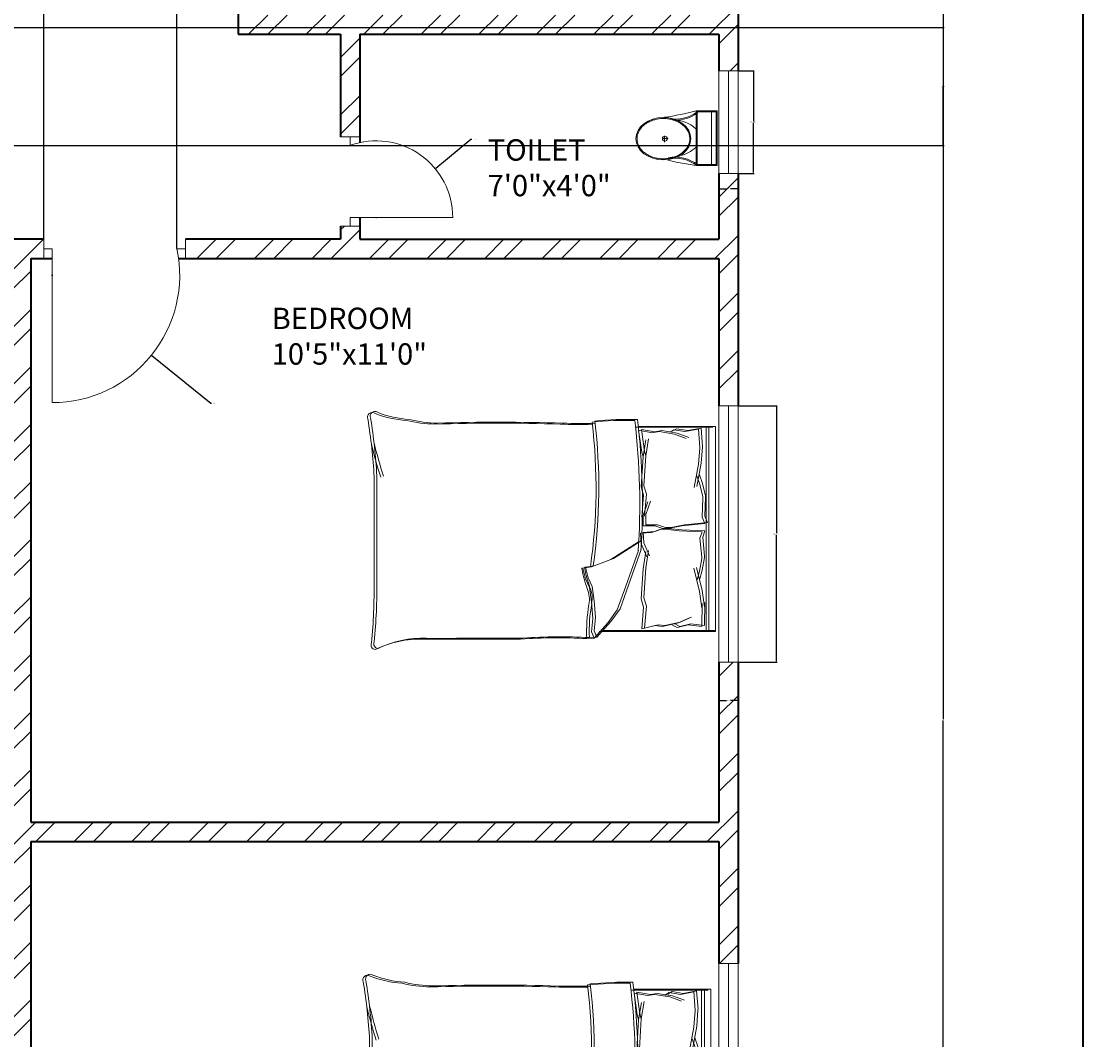
# Model space of a CAD drawing. Units: inches. Extents: x 2008 to 2657, y 1077 to 2165.
# Tile 14 of 16: x 2409 to 2657, y 1567 to 1805. Entities that reach past the tile are written whole.
import ezdxf

# ---------------------------------------------------------------- set-up
doc = ezdxf.new("R2010")
doc.units = ezdxf.units.IN
for name, color, linetype, lineweight in [('A-ANNO-DIMS', 2, 'Continuous', 18), ('A-ANNO-TTLB', 7, 'Continuous', 35), ('A-AREA-IDEN', 4, 'Continuous', 18), ('A-DOOR', 11, 'Continuous', 18), ('A-FLOR-FIXT', 8, 'Continuous', 18), ('A-FURN', 8, 'Continuous', 13), ('A-GLAZ', 191, 'Continuous', 18), ('A-WALL', 7, 'Continuous', 35)]:
    doc.layers.add(name, color=color, linetype=linetype, lineweight=lineweight)
doc.layers.add('A-WALL-PATT', color=30, linetype='Continuous', lineweight=13, true_color=0xf8991e)
doc.styles.get("Standard").update_dxf_attribs({"font": 'arial.ttf'})
doc.dimstyles.get("Standard").update_dxf_attribs({"dimtxt": 0.18, "dimasz": 0.18, "dimexe": 0.18, "dimexo": 0.0625, "dimgap": 0.09, "dimtad": 0, "dimtih": 1, "dimtoh": 1, "dimdec": 4, "dimzin": 0, "dimdsep": 46, "dimtxsty": 'Standard', "dimcen": 0.09, "dimadec": 0, "dimazin": 0, "dimtfac": 1, "dimtdec": 4, "dimtofl": 0, "dimtmove": 0, "dimatfit": 3, "dimfxl": 1, "dimtolj": 1, "dimtzin": 0, "dimarcsym": 0})

# ---------------------------------------------------------------- blocks, each defined once
blk = doc.blocks.new('A$C31115884')
for p, q in [((258, 466), (258, 523)), ((283, 498), (223, 498)), ((0, 200), (0, 0)), ((520, 200), (0, 200)), ((10, 190), (10, 10)), ((510, 190), (10, 190)), ((510, 10), (510, 190)), ((520, 0), (520, 200)), ((510, 54), (0, 54)), ((10, 10), (510, 10)), ((0, 0), (520, 0))]:
    blk.add_line(p, q)
blk.add_circle((256, 496), 23.6)
for centre, radius, start, end in [((2778, -205), 2807, 165.4549, 171.7133), ((-295, 403), 365, 324.2091, 9.3499), ((-295, 403), 375, 324.2091, 9.3499), ((139, 406), 293, 315.8436, 2.6563), ((806, 403), 375, 179.2036, 215.7909), ((806, 403), 365, 170.6501, 215.7909), ((3237, 905), 2807, 188.2867, 194.5451), ((384, 406), 293, 190.2774, 224.1564)]:
    blk.add_arc(centre, radius, start, end)
blk.add_ellipse((256, 510), major_axis=(0, -261), ratio=0.772727)
blk.add_open_spline([(256, 259), (263, 259), (270, 260), (288, 262), (299, 265), (320, 273), (330, 278), (350, 291), (360, 299), (378, 316), (386, 326), (402, 347), (409, 358), (421, 383), (427, 395), (436, 422), (440, 436), (445, 465), (447, 480), (448, 509), (448, 524), (445, 553), (443, 568), (436, 596), (432, 610), (422, 636), (416, 649), (402, 672), (395, 683), (379, 703), (370, 712), (351, 728), (341, 735), (321, 746), (310, 751), (289, 757), (278, 759), (256, 761), (245, 761), (223, 757), (212, 754), (191, 746), (181, 741), (161, 728), (151, 720), (133, 703), (125, 693), (110, 672), (103, 660), (90, 636), (85, 623), (76, 596), (72, 582), (67, 553), (66, 538), (64, 509), (65, 494), (68, 465), (70, 450), (77, 422), (81, 408), (91, 382), (97, 370), (111, 346), (118, 335), (135, 316), (144, 307), (162, 291), (172, 284), (193, 273), (203, 269), (225, 262), (236, 260), (250, 259), (253, 259), (256, 259)], degree=3, knots=[0, 0, 0, 0, 0.110105, 0.110105, 0.285049, 0.285049, 0.459994, 0.459994, 0.634938, 0.634938, 0.809882, 0.809882, 0.984827, 0.984827, 1.159771, 1.159771, 1.334715, 1.334715, 1.50966, 1.50966, 1.684604, 1.684604, 1.859549, 1.859549, 2.034493, 2.034493, 2.209437, 2.209437, 2.384382, 2.384382, 2.559326, 2.559326, 2.73427, 2.73427, 2.909215, 2.909215, 3.084159, 3.084159, 3.259103, 3.259103, 3.434048, 3.434048, 3.608992, 3.608992, 3.783936, 3.783936, 3.958881, 3.958881, 4.133825, 4.133825, 4.30877, 4.30877, 4.483714, 4.483714, 4.658658, 4.658658, 4.833603, 4.833603, 5.008547, 5.008547, 5.183491, 5.183491, 5.358436, 5.358436, 5.53338, 5.53338, 5.708324, 5.708324, 5.883269, 5.883269, 6.058213, 6.058213, 6.233158, 6.233158, 6.283185, 6.283185, 6.283185, 6.283185])
blk = doc.blocks.new('BED-DOUBLE')
for p, q in [((27.75, 52.87), (24.5, 49.16)), ((27.75, 52.87), (24.5, 49.16)), ((28.39, 53.1), (25.14, 49.39)), ((28.39, 53.1), (25.14, 49.39)), ((29.49, 52.95), (27.75, 52.87, 3.87)), ((29.49, 52.95), (27.75, 52.87, 3.87)), ((28.37, 51.33), (27.75, 52.87)), ((28.37, 51.33), (27.75, 52.87)), ((30.13, 53.18), (28.39, 53.1, 3.87)), ((30.13, 53.18), (28.39, 53.1, 3.87)), ((29, 51.56), (28.39, 53.1)), ((29, 51.56), (28.39, 53.1)), ((0, 51.49), (0.64, 51.49)), ((0, 3.48), (0, 51.49)), ((0, 51.27), (26.61, 51.27)), ((0, 51.27), (26.61, 51.27)), ((0.64, 51.49), (27.25, 51.49)), ((0.64, 51.49), (27.25, 51.49)), ((1.53, 3.48), (1.53, 51.27)), ((1.53, 3.48), (1.53, 51.27)), ((2.17, 3.7), (2.17, 51.49)), ((2.17, 3.7), (2.17, 51.49)), ((2.56, 50.11), (2.46, 44.71)), ((2.56, 50.11), (2.46, 44.71)), ((2.56, 50.11), (5.77, 49.73)), ((2.56, 50.11), (5.77, 49.73)), ((3.2, 50.34), (3.1, 44.94)), ((3.2, 50.34), (3.1, 44.94)), ((3.2, 50.34), (6.41, 49.96)), ((3.2, 50.34), (6.41, 49.96)), ((5.77, 49.73), (8.34, 50.33)), ((5.77, 49.73), (8.34, 50.33)), ((6.41, 49.96), (8.98, 50.56)), ((6.41, 49.96), (8.98, 50.56)), ((11.83, 50.11), (8.26, 49.31)), ((11.83, 50.11), (8.26, 49.31)), ((8.34, 50.33), (9.38, 49.82)), ((8.34, 50.33), (9.38, 49.81)), ((12.47, 50.34), (8.9, 49.54)), ((12.47, 50.34), (8.9, 49.54)), ((8.98, 50.56), (10.02, 50.04)), ((8.98, 50.56), (10.02, 50.04)), ((13.43, 49.92), (11.83, 50.11)), ((13.43, 49.92), (11.83, 50.11)), ((14.07, 50.15), (12.47, 50.34)), ((14.07, 50.15), (12.47, 50.34)), ((16.57, 50.7), (13.43, 49.92)), ((16.57, 50.7), (13.43, 49.92)), ((17.21, 50.93), (14.07, 50.15)), ((17.21, 50.93), (14.07, 50.15)), ((16.17, 45.57), (16.57, 50.7)), ((16.17, 45.57), (16.57, 50.7)), ((16.81, 45.8), (17.21, 50.93)), ((16.81, 45.8), (17.21, 50.93)), ((28.06, 48.23), (28.37, 51.33)), ((28.06, 48.23), (28.37, 51.33)), ((28.7, 48.46), (29, 51.56)), ((28.7, 48.46), (29, 51.56)), ((8.26, 49.31), (5.58, 48.13)), ((8.26, 49.31), (5.58, 48.13)), ((8.9, 49.54), (6.22, 48.36)), ((8.9, 49.54), (6.22, 48.36)), ((24.5, 49.16), (22.33, 46.22)), ((24.5, 49.16), (22.33, 46.22)), ((25.14, 49.39), (22.97, 46.45)), ((25.14, 49.39), (22.97, 46.45)), ((28.37, 44.36), (28.06, 48.23)), ((28.37, 44.36), (28.06, 48.23)), ((29, 44.59), (28.7, 48.46)), ((29, 44.59), (28.7, 48.46)), ((2.46, 44.71), (2.54, 45.71)), ((2.46, 44.71), (2.54, 45.71)), ((2.54, 45.71), (3.07, 41.91)), ((2.54, 45.71), (3.07, 41.91)), ((3.1, 44.94), (3.18, 45.94)), ((3.1, 44.94), (3.18, 45.94)), ((3.18, 45.94), (3.71, 42.14)), ((3.18, 45.94), (3.71, 42.14)), ((16.73, 43.61), (16.17, 45.57)), ((16.73, 43.61), (16.17, 45.57)), ((17.37, 43.84), (16.81, 45.8)), ((17.37, 43.83), (16.81, 45.8)), ((22.33, 46.22), (20.32, 40.64)), ((22.33, 46.22), (20.32, 40.64)), ((22.97, 46.45), (20.96, 40.87)), ((22.97, 46.45), (20.96, 40.87)), ((16.3, 36.6), (16.73, 43.61)), ((16.3, 36.6), (16.73, 43.61)), ((16.93, 36.83), (17.37, 43.84)), ((16.93, 36.82), (17.37, 43.83)), ((28.83, 40.95), (28.37, 44.36)), ((28.83, 40.95), (28.37, 44.36)), ((29.47, 41.18), (29, 44.59)), ((29.47, 41.18), (29, 44.59)), ((3.07, 41.91), (4.42, 36.5)), ((3.07, 41.91), (4.42, 36.5)), ((3.71, 42.14), (5.06, 36.72)), ((3.71, 42.14), (5.06, 36.72)), ((20.32, 40.64), (17.38, 32.31)), ((20.32, 40.64), (17.38, 32.31)), ((20.96, 40.87), (18.02, 32.54)), ((20.96, 40.87), (18.02, 32.53)), ((29.76, 38.94), (28.83, 40.95)), ((29.76, 38.94), (28.83, 40.95)), ((30.4, 39.17), (29.47, 41.18)), ((30.4, 39.17), (29.47, 41.18)), ((79.88, 15.29), (79.88, 39.91)), ((79.88, 15.29), (79.88, 39.91)), ((3.67, 39.2), (3.08, 37.14)), ((3.67, 39.2), (3.08, 37.14)), ((3.72, 37.36), (3.18, 34.43)), ((3.72, 37.36), (3.18, 34.43)), ((4.31, 39.43), (3.72, 37.36)), ((4.31, 39.43), (3.72, 37.36)), ((30.38, 36.46), (29.76, 38.94)), ((30.38, 36.46), (29.76, 38.94)), ((31.02, 36.69), (30.4, 39.17)), ((31.02, 36.69), (30.4, 39.17)), ((79.25, 15.06), (79.25, 39.68)), ((79.25, 15.06), (79.25, 39.68)), ((3.08, 37.14), (2.54, 34.21)), ((3.08, 37.14), (2.54, 34.2)), ((15.63, 32.56), (16.3, 36.6)), ((15.63, 32.56), (16.3, 36.6)), ((16.27, 32.79), (16.93, 36.83)), ((16.27, 32.79), (16.93, 36.82)), ((23.88, 34.45), (28.37, 36.15)), ((23.88, 34.45), (28.37, 36.15)), ((24.52, 34.68), (29, 36.38)), ((24.52, 34.68), (29, 36.38)), ((28.37, 36.15), (30.38, 36.46)), ((28.37, 36.15), (30.38, 36.46)), ((29, 36.38), (31.02, 36.69)), ((29, 36.38), (31.02, 36.69)), ((2.54, 34.21), (2.56, 33.88)), ((2.54, 34.2), (2.56, 33.88)), ((2.56, 33.88), (2.98, 29.46)), ((2.56, 33.88), (2.98, 29.46)), ((3.18, 34.43), (3.2, 34.11)), ((3.18, 34.43), (3.2, 34.11)), ((3.2, 34.11), (3.62, 29.68)), ((3.2, 34.11), (3.62, 29.68)), ((16.74, 30.75), (15.45, 33.82)), ((16.74, 30.75), (15.45, 33.82)), ((17.38, 30.98), (16.09, 34.05)), ((17.38, 30.98), (16.09, 34.05)), ((17.38, 30.26), (23.88, 34.45)), ((17.38, 30.26), (23.88, 34.45)), ((18.02, 30.49), (24.52, 34.68)), ((18.02, 30.49), (24.52, 34.68)), ((16.89, 28.3), (16.74, 30.75)), ((16.89, 28.3), (16.74, 30.75)), ((17.53, 28.53), (17.38, 30.98)), ((17.53, 28.53), (17.38, 30.98)), ((2.98, 29.46), (2.49, 27.98)), ((2.98, 29.46), (2.49, 27.98)), ((2.49, 27.98), (7.87, 27.73)), ((2.49, 27.98), (7.87, 27.73)), ((3.62, 29.68), (3.13, 28.21)), ((3.62, 29.68), (3.13, 28.21)), ((3.13, 28.21), (8.51, 27.96)), ((3.13, 28.21), (8.51, 27.96)), ((7.86, 26.79), (11.04, 27.37)), ((7.86, 26.79), (11.04, 27.37)), ((7.87, 27.73), (11.08, 27.36)), ((7.87, 27.73), (11.08, 27.36)), ((8.51, 27.96), (11.72, 27.58)), ((8.51, 27.96), (11.72, 27.58)), ((11.04, 27.37), (12.34, 27.37)), ((11.04, 27.37), (12.34, 27.37)), ((11.08, 27.36), (12.38, 27.44)), ((11.08, 27.36), (12.38, 27.44)), ((11.72, 27.58), (13.02, 27.66)), ((11.72, 27.58), (13.02, 27.66)), ((12.34, 27.37), (14.22, 26.79)), ((12.34, 27.37), (14.22, 26.79)), ((12.38, 27.44), (14.22, 28.13)), ((12.38, 27.44), (14.22, 28.13)), ((13.02, 27.66), (14.86, 28.36)), ((13.02, 27.66), (14.86, 28.36)), ((14.22, 28.13), (16.89, 28.3)), ((14.22, 28.13), (16.89, 28.3)), ((14.86, 28.36), (17.53, 28.53)), ((14.86, 28.36), (17.53, 28.53)), ((1.87, 25.98), (7.22, 26.56)), ((1.87, 25.98), (7.22, 26.56)), ((2.45, 24.54), (1.87, 25.98)), ((2.45, 24.54), (1.87, 25.98)), ((2.51, 26.21), (7.86, 26.79)), ((2.51, 26.21), (7.86, 26.79)), ((3.09, 24.77), (2.51, 26.21)), ((3.09, 24.77), (2.51, 26.21)), ((7.22, 26.56), (10.4, 27.14)), ((7.22, 26.56), (10.4, 27.14)), ((10.4, 27.14), (11.7, 27.14)), ((10.4, 27.14), (11.7, 27.14)), ((11.7, 27.14), (13.58, 26.56)), ((11.7, 27.14), (13.58, 26.56)), ((13.58, 26.56), (16.26, 26.56)), ((13.58, 26.56), (16.26, 26.56)), ((14.22, 26.79), (16.9, 26.79)), ((14.22, 26.79), (16.9, 26.79)), ((16.26, 26.56), (16.26, 24.1)), ((16.26, 26.56), (16.26, 24.1)), ((16.9, 26.79), (16.9, 24.33)), ((16.9, 26.79), (16.9, 24.33)), ((2.3, 20.09), (2.45, 24.54)), ((2.3, 20.09), (2.45, 24.54)), ((2.94, 20.32), (3.09, 24.77)), ((2.94, 20.32), (3.09, 24.77)), ((16.26, 24.1), (15.17, 20.96)), ((16.26, 24.1), (15.17, 20.96)), ((16.9, 24.33), (15.81, 21.19)), ((16.9, 24.33), (15.81, 21.19)), ((16.17, 19.38), (16.57, 24.52)), ((16.17, 19.38), (16.57, 24.52)), ((16.81, 19.61), (17.21, 24.74)), ((16.81, 19.61), (17.21, 24.74)), ((2.3, 19.77), (2.3, 20.09)), ((2.3, 19.77), (2.3, 20.09)), ((2.94, 20), (2.94, 20.32)), ((2.94, 20), (2.94, 20.32)), ((3.67, 17.11), (2.94, 20)), ((3.67, 17.11), (2.94, 20)), ((3.03, 16.88), (2.3, 19.77)), ((3.03, 16.88), (2.3, 19.77)), ((3.32, 12.11), (4.33, 17.6)), ((3.32, 12.11), (4.33, 17.6)), ((3.96, 12.34), (4.97, 17.83)), ((3.96, 12.34), (4.97, 17.83)), ((16.73, 17.42), (16.17, 19.38)), ((16.73, 17.42), (16.17, 19.38)), ((16.3, 10.41), (16.73, 17.42)), ((16.3, 10.41), (16.73, 17.42)), ((17.37, 17.65), (16.81, 19.61)), ((17.37, 17.65), (16.81, 19.61)), ((16.93, 10.64), (17.37, 17.65)), ((16.93, 10.64), (17.37, 17.65)), ((3.75, 14.86), (3.03, 16.88)), ((3.75, 14.86), (3.03, 16.88)), ((4.39, 15.08), (3.67, 17.11)), ((4.39, 15.08), (3.67, 17.11)), ((3.03, 8.29), (3.32, 12.11)), ((3.03, 8.29), (3.32, 12.11)), ((3.67, 8.51), (3.96, 12.34)), ((3.67, 8.51), (3.96, 12.34)), ((15.63, 6.38), (16.3, 10.41)), ((15.63, 6.38), (16.3, 10.41)), ((16.27, 6.61), (16.93, 10.64)), ((16.27, 6.61), (16.93, 10.64)), ((16.3, 10.41), (16.62, 9.28)), ((16.3, 10.41), (16.62, 9.28)), ((16.93, 10.64), (17.26, 9.51)), ((16.93, 10.64), (17.26, 9.51)), ((3.01, 8.18), (3.03, 8.29)), ((3.01, 8.18), (3.03, 8.29)), ((3.34, 3.9), (3.01, 8.18)), ((3.34, 3.9), (3.01, 8.18)), ((3.65, 8.41), (3.67, 8.51)), ((3.65, 8.41), (3.67, 8.51)), ((3.98, 4.13), (3.65, 8.41)), ((3.98, 4.13), (3.65, 8.41)), ((16.62, 9.28), (17.34, 4.18)), ((16.62, 9.28), (17.34, 4.18)), ((17.26, 9.51), (17.98, 4.41)), ((17.26, 9.51), (17.98, 4.41)), ((8.96, 5.05), (6.21, 6.06)), ((8.96, 5.05), (6.21, 6.06)), ((9.59, 5.28), (6.85, 6.29)), ((9.59, 5.28), (6.85, 6.29)), ((12.57, 4.47), (8.96, 5.05)), ((12.57, 4.47), (8.96, 5.05)), ((13.21, 4.7), (9.59, 5.28)), ((13.21, 4.7), (9.59, 5.28)), ((14.8, 4.99), (13.21, 4.7)), ((14.8, 4.99), (13.21, 4.7)), ((17.98, 4.41), (14.8, 4.99)), ((17.98, 4.41), (14.8, 4.99)), ((18.11, 3.48), (0, 3.48)), ((18.11, 3.48), (0, 3.48)), ((18.75, 3.7), (0.64, 3.7)), ((18.75, 3.7), (0.64, 3.7)), ((3.32, 3.9), (6.5, 4.47)), ((3.32, 3.89), (6.5, 4.47)), ((3.96, 4.12), (7.14, 4.7)), ((3.96, 4.12), (7.14, 4.7)), ((6.5, 4.47), (9.1, 4.04)), ((6.5, 4.47), (9.1, 4.04)), ((7.14, 4.7), (9.74, 4.27)), ((7.14, 4.7), (9.74, 4.27)), ((9.1, 4.04), (10.11, 4.62)), ((9.1, 4.04), (10.11, 4.62)), ((9.74, 4.27), (10.75, 4.85)), ((9.74, 4.27), (10.75, 4.85)), ((14.16, 4.76), (12.57, 4.47)), ((14.16, 4.76), (12.57, 4.47)), ((17.34, 4.18), (14.16, 4.76)), ((17.34, 4.18), (14.16, 4.76))]:
    blk.add_line(p, q)
for centre, radius, start, end in [((68.67, 76.16), 23.07, 267.4714, 296.4681), ((68.67, 76.16), 23.07, 267.4714, 296.4681), ((69.31, 76.39), 23.07, 267.4714, 296.4681), ((69.31, 76.39), 23.07, 267.4714, 296.4681), ((78.87, 54.41), 1.1, 332.6588, 86.02), ((78.87, 54.41), 1.1, 332.6588, 86.02), ((79.51, 54.64), 1.1, 332.6588, 86.02), ((79.51, 54.64), 1.1, 332.6588, 86.02), ((-6.66, 51.33), 36.18, 349.8763, 2.5657), ((-6.66, 51.33), 36.18, 349.8763, 2.5657), ((36.32, 182.27), 129.5, 266.9791, 273.8365), ((36.32, 182.27), 129.5, 266.9791, 273.8365), ((-6.02, 51.56), 36.18, 349.8763, 2.5657), ((-6.02, 51.56), 36.18, 349.8763, 2.5657), ((36.95, 182.49), 129.5, 266.9791, 273.8365), ((36.95, 182.49), 129.5, 266.9791, 273.8365), ((67.82, -4508.74), 4561.86, 90.00217, 90.28689), ((67.82, -4508.74), 4561.86, 90.00217, 90.28689), ((68.46, -4508.51), 4561.86, 90.00217, 90.28689), ((68.46, -4508.51), 4561.86, 90.00217, 90.28689), ((212.28, 41.15), 133.04, 174.4998, 180.6351), ((212.28, 41.15), 133.04, 174.4998, 180.6351), ((212.92, 41.38), 133.04, 174.4998, 180.6351), ((212.92, 41.38), 133.04, 174.4998, 180.6351), ((35.07, 43.74), 6.22, 168.6608, 203.7384), ((35.07, 43.74), 6.22, 168.6608, 203.7384), ((35.71, 43.97), 6.22, 168.6608, 203.7384), ((35.71, 43.97), 6.22, 168.6608, 203.7384), ((1.48, 31.15), 29.65, 10.6617, 19.8806), ((1.48, 31.15), 29.65, 10.6617, 19.8806), ((2.12, 31.38), 29.65, 10.6617, 19.8806), ((2.12, 31.38), 29.65, 10.6617, 19.8806), ((156.32, 17.76), 129.02, 171.7845, 186.9006), ((156.32, 17.76), 129.02, 171.7845, 186.9006), ((156.96, 17.98), 129.02, 171.7845, 186.9006), ((156.96, 17.98), 129.02, 171.7845, 186.9006), ((30.44, 36.64), 0.185, 250.2464, 1.1377), ((30.44, 36.64), 0.185, 250.2464, 1.1377), ((31.08, 36.87), 0.185, 250.2464, 1.1377), ((31.08, 36.86), 0.185, 250.2464, 1.1377), ((182.05, 21.36), 164.97, 176.0865, 186.7821), ((182.05, 21.36), 164.97, 176.0865, 186.7821), ((182.69, 21.59), 164.97, 176.0865, 186.7821), ((182.69, 21.59), 164.97, 176.0865, 186.7821), ((-23.71, -17.22), 106.46, 13.3832, 17.7053), ((-23.71, -17.22), 106.46, 13.3832, 17.7053), ((-23.07, -16.99), 106.46, 13.3832, 17.7053), ((-23.07, -16.99), 106.46, 13.3832, 17.7053), ((200.84, 21.43), 121.76, 182.9958, 189.4091), ((200.84, 21.43), 121.76, 182.9958, 189.4091), ((201.48, 21.66), 121.76, 182.9958, 189.4091), ((201.48, 21.66), 121.76, 182.9958, 189.4091), ((31.17, -167.31), 170.11, 88.4762, 91.0082), ((31.17, -167.31), 170.11, 88.4762, 91.0082), ((31.81, -167.08), 170.11, 88.4762, 91.0082), ((31.81, -167.08), 170.11, 88.4762, 91.0082), ((50.61, 484.82), 482.31, 268.2277, 271.7185), ((50.61, 484.82), 482.31, 268.2277, 271.7185), ((51.25, 485.05), 482.31, 268.2277, 271.7185), ((51.25, 485.05), 482.31, 268.2277, 271.7185), ((64.52, -26.9), 29.63, 76.0648, 88.9113), ((64.52, -26.9), 29.63, 76.0648, 88.9113), ((65.15, -26.67), 29.63, 76.0648, 88.9113), ((65.15, -26.67), 29.63, 76.0648, 88.9113), ((20.1, 85.16), 83.31, 268.7218, 275.604), ((20.1, 85.16), 83.31, 268.7218, 275.604), ((20.74, 85.39), 83.31, 268.7218, 275.604), ((20.74, 85.39), 83.31, 268.7218, 275.604), ((70.28, -21.66), 23.56, 67.9751, 86.652), ((70.28, -21.66), 23.56, 67.9751, 86.652), ((70.92, -21.43), 23.56, 67.9751, 86.652), ((70.92, -21.43), 23.56, 67.9751, 86.652), ((79.72, 1.09), 1.09, 236.1736, 23.4781), ((79.72, 1.09), 1.09, 236.1736, 23.4781), ((80.36, 1.32), 1.09, 236.1736, 23.4781), ((80.36, 1.32), 1.09, 236.1736, 23.4781)]:
    blk.add_arc(centre, radius, start, end)
blk = doc.blocks.new('WIN-60IN-B')
for p, q in [((0, 4.5), (0, 0)), ((0, 4.5), (60, 4.5)), ((60, 2.25), (60, 4.5)), ((60, 4.5), (60, 0)), ((0, 0), (0, 2.25)), ((0, 2.25), (60, 2.25)), ((60, 0), (0, 0))]:
    blk.add_line(p, q)
blk = doc.blocks.new('WIN-24IN-A')
for p, q in [((0, 24), (4.5, 24)), ((0, 0), (0, 24)), ((4.5, 24), (2.25, 24)), ((2.25, 24), (2.25, 0)), ((4.5, 24), (4.5, 0)), ((4.5, 0), (0, 0)), ((2.25, 0), (4.5, 0))]:
    blk.add_line(p, q)
blk = doc.blocks.new('WIN-60IN-A')
for p, q in [((0, 60), (4.5, 60)), ((0, 60), (0, 0)), ((4.5, 60), (2.25, 60)), ((2.25, 60), (2.25, 0)), ((4.5, 0), (4.5, 60)), ((4.5, 0), (0, 0)), ((2.25, 0), (4.5, 0))]:
    blk.add_line(p, q)
blk = doc.blocks.new('*D21')
at = {"layer": 'A-ANNO-DIMS', "color": 0, "lineweight": -2, "transparency": 16777216}
for p, q in [((2576.82, 1715.18), (2585.94, 1715.18)), ((2585.76, 1715), (2585.76, 1685.37)), ((2585.76, 1655.36), (2585.76, 1685)), ((2576.82, 1655.18), (2585.94, 1655.18))]:
    blk.add_line(p, q, dxfattribs=at)
at = {"layer": 'A-ANNO-DIMS', "color": 0, "transparency": 16777216}
for points in [[(2585.73, 1715), (2585.79, 1715), (2585.76, 1715.18)], [(2585.73, 1655.36), (2585.79, 1655.36), (2585.76, 1655.18)]]:
    blk.add_solid(points, dxfattribs=at)
at = {"layer": 'Defpoints', "color": 0, "transparency": 16777216}
for p in [(2576.76, 1715.18), (2585.76, 1715.18), (2576.76, 1655.18)]:
    blk.add_point(p, dxfattribs=at)
at = {"layer": 'A-ANNO-DIMS', "color": 0, "transparency": 16777216, "insert": (2585.76, 1685.18), "char_height": 0.18, "attachment_point": 5}
blk.add_mtext('\\A1;WIN A 60 TYP.', dxfattribs=at)
blk = doc.blocks.new('*D22')
at = {"layer": 'A-ANNO-DIMS', "color": 0, "lineweight": -2, "transparency": 16777216}
for p, q in [((2572.26, 1655.12), (2572.26, 1646)), ((2576.76, 1655.12), (2576.76, 1646)), ((2572.44, 1646.18), (2574.05, 1646.18)), ((2576.58, 1646.18), (2574.97, 1646.18))]:
    blk.add_line(p, q, dxfattribs=at)
at = {"layer": 'A-ANNO-DIMS', "color": 0, "transparency": 16777216}
for points in [[(2572.44, 1646.21), (2572.44, 1646.15), (2572.26, 1646.18)], [(2576.58, 1646.21), (2576.58, 1646.15), (2576.76, 1646.18)]]:
    blk.add_solid(points, dxfattribs=at)
at = {"layer": 'Defpoints', "color": 0, "transparency": 16777216}
for p in [(2572.26, 1655.18), (2576.76, 1655.18), (2576.76, 1646.18)]:
    blk.add_point(p, dxfattribs=at)
at = {"layer": 'A-ANNO-DIMS', "color": 0, "transparency": 16777216, "insert": (2574.51, 1646.18), "char_height": 0.18, "attachment_point": 5}
blk.add_mtext('\\A1;5 TYP.', dxfattribs=at)
blk = doc.blocks.new('*D25')
at = {"layer": 'A-ANNO-DIMS', "color": 0, "lineweight": -2, "transparency": 16777216}
for p, q in [((2576.82, 1793.61), (2580.54, 1793.61)), ((2580.36, 1793.43), (2580.36, 1781.79)), ((2580.36, 1769.79), (2580.36, 1781.43)), ((2576.82, 1769.61), (2580.54, 1769.61))]:
    blk.add_line(p, q, dxfattribs=at)
at = {"layer": 'A-ANNO-DIMS', "color": 0, "transparency": 16777216}
for points in [[(2580.33, 1793.43), (2580.39, 1793.43), (2580.36, 1793.61)], [(2580.33, 1769.79), (2580.39, 1769.79), (2580.36, 1769.61)]]:
    blk.add_solid(points, dxfattribs=at)
at = {"layer": 'Defpoints', "color": 0, "transparency": 16777216}
for p in [(2576.76, 1793.61), (2580.36, 1793.61), (2576.76, 1769.61)]:
    blk.add_point(p, dxfattribs=at)
at = {"layer": 'A-ANNO-DIMS', "color": 0, "transparency": 16777216, "insert": (2580.36, 1781.61), "char_height": 0.18, "attachment_point": 5}
blk.add_mtext('\\A1;WIN A 24 TYP.', dxfattribs=at)
blk = doc.blocks.new('*D26')
at = {"layer": 'A-ANNO-DIMS', "color": 0, "lineweight": -2, "transparency": 16777216}
for p, q in [((2572.26, 1769.55), (2572.26, 1765.83)), ((2576.76, 1769.55), (2576.76, 1765.83)), ((2572.44, 1766.01), (2574.05, 1766.01)), ((2576.58, 1766.01), (2574.97, 1766.01))]:
    blk.add_line(p, q, dxfattribs=at)
at = {"layer": 'A-ANNO-DIMS', "color": 0, "transparency": 16777216}
for points in [[(2572.44, 1766.04), (2572.44, 1765.98), (2572.26, 1766.01)], [(2576.58, 1766.04), (2576.58, 1765.98), (2576.76, 1766.01)]]:
    blk.add_solid(points, dxfattribs=at)
at = {"layer": 'Defpoints', "color": 0, "transparency": 16777216}
for p in [(2572.26, 1769.61), (2576.76, 1769.61), (2576.76, 1766.01)]:
    blk.add_point(p, dxfattribs=at)
at = {"layer": 'A-ANNO-DIMS', "color": 0, "transparency": 16777216, "insert": (2574.51, 1766.01), "char_height": 0.18, "attachment_point": 5}
blk.add_mtext('\\A1;5 TYP.', dxfattribs=at)
blk = doc.blocks.new('*D32')
at = {"layer": 'A-ANNO-DIMS', "color": 0, "lineweight": -2, "transparency": 16777216}
for p, q in [((2576.82, 2094.67), (2624.99, 2094.67)), ((2624.81, 2094.49), (2624.81, 1641.86)), ((2624.81, 1188.85), (2624.81, 1641.49)), ((2576.82, 1188.67), (2624.99, 1188.67))]:
    blk.add_line(p, q, dxfattribs=at)
at = {"layer": 'A-ANNO-DIMS', "color": 0, "transparency": 16777216}
for points in [[(2624.78, 2094.49), (2624.84, 2094.49), (2624.81, 2094.67)], [(2624.78, 1188.85), (2624.84, 1188.85), (2624.81, 1188.67)]]:
    blk.add_solid(points, dxfattribs=at)
at = {"layer": 'Defpoints', "color": 0, "transparency": 16777216}
for p in [(2576.76, 2094.67), (2624.81, 2094.67), (2576.76, 1188.67)]:
    blk.add_point(p, dxfattribs=at)
at = {"layer": 'A-ANNO-DIMS', "color": 0, "transparency": 16777216, "insert": (2624.81, 1641.67), "char_height": 0.18, "attachment_point": 5}
blk.add_mtext('\\A1;906', dxfattribs=at)
blk = doc.blocks.new('*D57')
at = {"layer": 'A-ANNO-DIMS', "color": 0, "lineweight": -2, "transparency": 16777216}
for p, q in [((2414.28, 1754.24), (2414.28, 2142.9)), ((2414.46, 2142.72), (2429.47, 2142.72)), ((2445.27, 2142.72), (2430.26, 2142.72)), ((2445.45, 1751.99), (2445.45, 2142.9))]:
    blk.add_line(p, q, dxfattribs=at)
at = {"layer": 'A-ANNO-DIMS', "color": 0, "transparency": 16777216}
for points in [[(2414.46, 2142.75), (2414.46, 2142.69), (2414.28, 2142.72)], [(2445.27, 2142.75), (2445.27, 2142.69), (2445.45, 2142.72)]]:
    blk.add_solid(points, dxfattribs=at)
at = {"layer": 'Defpoints', "color": 0, "transparency": 16777216}
for p in [(2445.45, 2142.72), (2414.28, 1754.17), (2445.45, 1751.92)]:
    blk.add_point(p, dxfattribs=at)
at = {"layer": 'A-ANNO-DIMS', "color": 0, "transparency": 16777216, "insert": (2429.87, 2142.72), "char_height": 0.18, "attachment_point": 5}
blk.add_mtext('\\A1;31.17', dxfattribs=at)
blk = doc.blocks.new('*D65')
at = {"layer": 'A-ANNO-DIMS', "color": 0, "lineweight": -2, "transparency": 16777216}
for p, q in [((2323.2, 1803.79), (2624.99, 1803.79)), ((2624.81, 1803.61), (2624.81, 1790.13)), ((2624.81, 1776.29), (2624.81, 1789.77)), ((2323.2, 1776.11), (2624.99, 1776.11))]:
    blk.add_line(p, q, dxfattribs=at)
at = {"layer": 'A-ANNO-DIMS', "color": 0, "transparency": 16777216}
for points in [[(2624.78, 1803.61), (2624.84, 1803.61), (2624.81, 1803.79)], [(2624.78, 1776.29), (2624.84, 1776.29), (2624.81, 1776.11)]]:
    blk.add_solid(points, dxfattribs=at)
at = {"layer": 'Defpoints', "color": 0, "transparency": 16777216}
for p in [(2323.13, 1803.79), (2323.13, 1776.11), (2624.81, 1776.11)]:
    blk.add_point(p, dxfattribs=at)
at = {"layer": 'A-ANNO-DIMS', "color": 0, "transparency": 16777216, "insert": (2624.81, 1789.95), "char_height": 0.18, "attachment_point": 5}
blk.add_mtext('\\A1;27.684', dxfattribs=at)
blk = doc.blocks.new('*D70')
at = {"layer": 'A-ANNO-DIMS', "color": 0, "lineweight": -2, "transparency": 16777216}
for p, q in [((2416.19, 1745.74), (2416.37, 1745.74)), ((2416.28, 1745.65), (2416.28, 1745.83)), ((2453.35, 1715.71), (2439.59, 1726.86)), ((2453.53, 1715.71), (2453.35, 1715.71))]:
    blk.add_line(p, q, dxfattribs=at)
at = {"layer": 'A-ANNO-DIMS', "color": 0, "transparency": 16777216}
blk.add_solid([(2439.61, 1726.88), (2439.57, 1726.83), (2439.45, 1726.97)], dxfattribs=at)
at = {"layer": 'Defpoints', "color": 0, "transparency": 16777216}
for p in [(2416.28, 1745.74), (2439.45, 1726.97)]:
    blk.add_point(p, dxfattribs=at)
at = {"layer": 'A-ANNO-DIMS', "color": 0, "transparency": 16777216, "insert": (2454.01, 1715.71), "char_height": 0.18, "attachment_point": 5}
blk.add_mtext('\\A1;R29.82', dxfattribs=at)
blk = doc.blocks.new('*D90')
at = {"layer": 'A-ANNO-DIMS', "color": 0, "lineweight": -2, "transparency": 16777216}
for p, q in [((2514.25, 1777.51), (2506.07, 1770.78)), ((2514.43, 1777.51), (2514.25, 1777.51)), ((2491.97, 1759.27), (2492.15, 1759.27)), ((2492.06, 1759.18), (2492.06, 1759.36))]:
    blk.add_line(p, q, dxfattribs=at)
at = {"layer": 'A-ANNO-DIMS', "color": 0, "transparency": 16777216}
blk.add_solid([(2506.05, 1770.81), (2506.09, 1770.76), (2505.93, 1770.67)], dxfattribs=at)
at = {"layer": 'Defpoints', "color": 0, "transparency": 16777216}
for p in [(2505.93, 1770.67), (2492.06, 1759.27)]:
    blk.add_point(p, dxfattribs=at)
at = {"layer": 'A-ANNO-DIMS', "color": 0, "transparency": 16777216, "insert": (2514.98, 1777.51), "char_height": 0.18, "attachment_point": 5}
blk.add_mtext('\\A1;R17.955', dxfattribs=at)

msp = doc.modelspace()

# ---------------------------------------------------------------- hatches: boundary and pattern name
at = {"layer": 'A-WALL-PATT'}
h = msp.add_hatch(dxfattribs=at)
h.set_pattern_fill('ANSI32', color=256)
h.paths.add_polyline_path([(2109.2619, 2094.6743), (2104.7619, 2094.6743), (2104.7619, 2072.1743), (2104.7619, 2021.6151), (2109.2619, 2021.6151), (2109.2619, 2055.6743), (2126.1387, 2055.6743), (2126.1387, 2057.9243), (2126.1387, 2060.1743), (2109.2619, 2060.1743)])
h.paths.add_polyline_path([(2223.2494, 2057.9243), (2223.2494, 2060.1743), (2186.1387, 2060.1743), (2186.1387, 2055.6743), (2223.2494, 2055.6743)])
h.paths.add_polyline_path([(2250.7619, 2072.1743), (2250.7619, 2090.1743), (2250.7619, 2094.6743), (2246.2619, 2094.6743), (2246.2619, 2060.1743), (2242.7242, 2060.1743), (2242.7242, 2055.6743), (2246.2619, 2055.6743), (2246.2619, 1899.6743), (2242.7458, 1899.6743), (2242.7458, 1897.4243), (2242.7458, 1895.1743), (2246.2619, 1895.1743), (2246.2619, 1878.8745), (2248.5119, 1878.8745), (2250.7619, 1878.8745), (2250.7619, 1991.1743), (2250.7619, 2025.6743), (2257.6798, 2025.6743), (2257.6798, 2027.9243), (2257.6798, 2030.1743), (2250.7619, 2030.1743)])
h.paths.add_polyline_path([(2411.2619, 2031.6743), (2409.0119, 2031.6743), (2406.7619, 2031.6743), (2406.7619, 2030.1743), (2322.7619, 2030.1743), (2322.7619, 2053.3443), (2318.2619, 2053.3443), (2318.2619, 2030.1743), (2305.6798, 2030.1743), (2305.6798, 2025.6743), (2318.2619, 2025.6743), (2322.7619, 2025.6743), (2406.7619, 2025.6743), (2406.7619, 1995.6743), (2406.7619, 1847.2677), (2250.7619, 1847.2677), (2250.7619, 1850.9902), (2248.5119, 1850.9902), (2246.2619, 1850.9902), (2246.2619, 1847.1743), (2246.2619, 1842.7677), (2303.0015, 1842.7677), (2303.0015, 1667.2413), (2298.4208, 1667.2413), (2298.4208, 1662.7413), (2303.0015, 1662.7413), (2303.0015, 1649.8758), (2307.5015, 1649.8758), (2307.5015, 1842.7677), (2406.7619, 1842.7677), (2411.2619, 1842.7677), (2411.2619, 1878.6743), (2415.8196, 1878.6743), (2415.8196, 1880.9243), (2415.8196, 1883.1743), (2411.2619, 1883.1743)])
h.paths.add_polyline_path([(2411.2619, 2094.6743), (2406.7619, 2094.6743), (2318.2619, 2094.6743), (2318.2619, 2077.3443), (2322.7619, 2077.3443), (2322.7619, 2090.1743), (2406.7619, 2090.1743), (2406.7619, 2072.1743), (2406.7619, 2067.6743), (2406.7619, 2052.7524), (2411.2619, 2052.7524), (2411.2619, 2055.6743), (2414.9888, 2055.6743), (2414.9888, 2057.9243), (2414.9888, 2060.1743), (2411.2619, 2060.1743), (2411.2619, 2072.1743)])
h.paths.add_polyline_path([(2576.7619, 2072.1743), (2576.7619, 2094.6743), (2572.2619, 2094.6743), (2572.2619, 2060.1743), (2525.8113, 2060.1743), (2525.8113, 2055.6743), (2572.2619, 2055.6743), (2572.2619, 1994.289), (2576.7619, 1994.289)])
h.paths.add_polyline_path([(2465.8113, 2060.1743), (2436.2802, 2060.1743), (2436.2802, 2055.6743), (2465.8113, 2055.6743), (2465.8113, 2057.9243)])
h.paths.add_polyline_path([(2576.7619, 1934.289), (2574.5119, 1934.289), (2572.2619, 1934.289), (2572.2619, 1883.1743), (2447.7027, 1883.1743), (2447.7027, 1878.6743), (2459.7619, 1878.6743), (2459.7619, 1830.4982), (2464.2619, 1830.4982), (2464.2619, 1878.6743), (2572.2619, 1878.6743), (2572.2619, 1868.4883), (2576.7619, 1868.4883)])
h.paths.add_polyline_path([(2576.7619, 1832.4883), (2572.2619, 1832.4883), (2572.2619, 1806.6743), (2464.2619, 1806.6743), (2464.2619, 1809.6629), (2459.7619, 1809.6629), (2459.7619, 1802.1743), (2483.7619, 1802.1743), (2483.7619, 1778.1743), (2488.2619, 1778.1743), (2488.2619, 1802.1743), (2572.2619, 1802.1743), (2572.2619, 1793.6101), (2576.7619, 1793.6101)])
h.paths.add_polyline_path([(2576.7619, 1769.6101), (2572.2619, 1769.6101), (2572.2619, 1754.1743), (2488.2619, 1754.1743), (2488.2619, 1757.2675), (2486.0119, 1757.2675), (2483.7619, 1757.2675), (2483.7619, 1754.1743), (2447.4528, 1754.1743), (2447.4528, 1749.6743), (2483.7619, 1749.6743), (2572.2619, 1749.6743), (2572.2619, 1715.1837), (2576.7619, 1715.1837)])
h.paths.add_polyline_path([(2576.7619, 1655.1837), (2572.2619, 1655.1837), (2572.2619, 1617.6743), (2411.2619, 1617.6743), (2411.2619, 1749.6743), (2414.2827, 1749.6743), (2414.2827, 1754.1743), (2406.7619, 1754.1743), (2406.7619, 1749.6743), (2406.7619, 1617.6743), (2307.5015, 1617.6743), (2307.5015, 1621.0007), (2305.2515, 1621.0007), (2303.0015, 1621.0007), (2303.0015, 1609.6944), (2307.5015, 1609.6944), (2307.5015, 1613.1743), (2406.7619, 1613.1743), (2406.7619, 1476.6743), (2415.532, 1476.6743), (2415.532, 1478.9243), (2415.532, 1481.1743), (2411.2619, 1481.1743), (2411.2619, 1613.1743), (2572.2619, 1613.1743), (2572.2619, 1584.6086), (2576.7619, 1584.6086)])
h.paths.add_polyline_path([(2576.7619, 1524.6086), (2572.2619, 1524.6086), (2572.2619, 1481.1743), (2483.7619, 1481.1743), (2447.5119, 1481.1743), (2447.5119, 1476.6743), (2483.7619, 1476.6743), (2483.7619, 1473.5051), (2488.2619, 1473.5051), (2488.2619, 1476.6743), (2572.2619, 1476.6743), (2572.2619, 1469.5488), (2576.7619, 1469.5488)])
h.paths.add_polyline_path([(2576.7619, 1445.5488), (2572.2619, 1445.5488), (2572.2619, 1428.6743), (2488.2619, 1428.6743), (2488.2619, 1455.6743), (2486.0119, 1455.6743), (2483.7619, 1455.6743), (2483.7619, 1428.6743), (2459.7619, 1428.6743), (2459.7619, 1422.1519), (2464.2619, 1422.1519), (2464.2619, 1424.1743), (2572.2619, 1424.1743), (2572.2619, 1407.5685), (2576.7619, 1407.5685)])
h.paths.add_polyline_path([(2576.7619, 1371.5685), (2572.2619, 1371.5685), (2572.2619, 1352.1743), (2464.2619, 1352.1743), (2464.2619, 1403.1384), (2462.0119, 1403.1384), (2459.7619, 1403.1384), (2459.7619, 1352.1743), (2446.3194, 1352.1743), (2446.3194, 1347.6743), (2572.2619, 1347.6743), (2572.2619, 1321.0291), (2576.7619, 1321.0291)])
h.paths.add_polyline_path([(2462.703, 1227.6743), (2436.0298, 1227.6743), (2436.0298, 1225.4243), (2436.0298, 1223.1743), (2462.703, 1223.1743), (2462.703, 1225.4243)])
h.paths.add_polyline_path([(2576.7619, 1261.0291), (2574.5119, 1261.0291), (2572.2619, 1261.0291), (2572.2619, 1227.6743), (2522.703, 1227.6743), (2522.703, 1223.1743), (2572.2619, 1223.1743), (2572.2619, 1188.6743), (2576.7619, 1188.6743), (2576.7619, 1193.1743), (2576.7619, 1223.1743)])
h.paths.add_polyline_path([(2414.2823, 1227.6743), (2411.2619, 1227.6743), (2411.2619, 1267.1779), (2409.0119, 1267.1779), (2406.7619, 1267.1779), (2406.7619, 1227.6743), (2322.7619, 1227.6743), (2322.7619, 1244.3623), (2318.2619, 1244.3623), (2318.2619, 1223.1743), (2406.7619, 1223.1743), (2406.7619, 1193.1743), (2406.7619, 1188.6743), (2411.2619, 1188.6743), (2411.2619, 1193.1743), (2411.2619, 1223.1743), (2414.2823, 1223.1743)])
h.paths.add_polyline_path([(2411.2619, 1347.6743), (2414.702, 1347.6743), (2414.702, 1349.9243), (2414.702, 1352.1743), (2411.2619, 1352.1743), (2411.2619, 1416.7413), (2307.5015, 1416.7413), (2307.5015, 1579.8489), (2305.2515, 1579.8489), (2303.0015, 1579.8489), (2303.0015, 1566.7413), (2299.2719, 1566.7413), (2299.2719, 1562.2413), (2303.0015, 1562.2413), (2303.0015, 1416.7413), (2246.2619, 1416.7413), (2246.2619, 1409.8616), (2250.7619, 1409.8616), (2250.7619, 1412.2413), (2406.7619, 1412.2413), (2406.7619, 1292.1743), (2304.9703, 1292.1743), (2304.9703, 1287.6743), (2318.2619, 1287.6743), (2318.2619, 1268.3623), (2322.7619, 1268.3623), (2322.7619, 1287.6743), (2406.7619, 1287.6743), (2406.7619, 1285.4748), (2411.2619, 1285.4748)])
h.paths.add_polyline_path([(2109.2619, 1262.7482), (2104.7619, 1262.7482), (2104.7619, 1223.1743), (2104.7619, 1193.1743), (2104.7619, 1188.6743), (2109.2619, 1188.6743), (2109.2619, 1223.1743), (2126.7928, 1223.1743), (2126.7928, 1225.4243), (2126.7928, 1227.6743), (2109.2619, 1227.6743)])
h.paths.add_polyline_path([(2222.3268, 1227.6743), (2186.7928, 1227.6743), (2186.7928, 1223.1743), (2222.3268, 1223.1743)])
h.paths.add_polyline_path([(2250.7619, 1287.6743), (2256.9703, 1287.6743), (2256.9703, 1289.9243), (2256.9703, 1292.1743), (2250.7619, 1292.1743), (2250.7619, 1382.2078), (2248.5119, 1382.2078), (2246.2619, 1382.2078), (2246.2619, 1347.6743), (2246.2619, 1227.6743), (2242.6068, 1227.6743), (2242.6068, 1223.1743), (2246.2619, 1223.1743), (2246.2619, 1188.6743), (2250.7619, 1188.6743), (2250.7619, 1193.1743), (2250.7619, 1227.6743)])
h.paths.add_polyline_path([(2133.2619, 1349.9243), (2133.2619, 1352.1743), (2109.2619, 1352.1743), (2109.2619, 1375.2826), (2104.7619, 1375.2826), (2104.7619, 1322.7482), (2109.2619, 1322.7482), (2109.2619, 1347.6743), (2133.2619, 1347.6743)])
h.paths.add_polyline_path([(2210.2105, 1352.1743), (2161.7619, 1352.1743), (2161.7619, 1412.2413), (2185.7619, 1412.2413), (2185.7619, 1420.1851), (2183.5119, 1420.1851), (2181.2619, 1420.1851), (2181.2619, 1416.7413), (2109.2619, 1416.7413), (2109.2619, 1452.4006), (2104.7619, 1452.4006), (2104.7619, 1399.2826), (2109.2619, 1399.2826), (2109.2619, 1412.2413), (2157.2619, 1412.2413), (2157.2619, 1352.1743), (2154.3383, 1352.1743), (2154.3383, 1347.6743), (2210.2105, 1347.6743)])
h.paths.add_polyline_path([(2185.7619, 1514.2413), (2161.7619, 1514.2413), (2161.7619, 1518.1307), (2159.5119, 1518.1307), (2157.2619, 1518.1307), (2157.2619, 1514.2413), (2109.2619, 1514.2413), (2109.2619, 1528.997), (2107.0119, 1528.997), (2104.7619, 1528.997), (2104.7619, 1488.4006), (2109.2619, 1488.4006), (2109.2619, 1509.7413), (2181.2619, 1509.7413), (2181.2619, 1441.2042), (2185.7619, 1441.2042)])
h.paths.add_polyline_path([(2270.4025, 1566.7413), (2109.2619, 1566.7413), (2080.7619, 1566.7413), (2080.7619, 1586.5643), (2076.2619, 1586.5643), (2076.2619, 1562.2413), (2080.7619, 1562.2413), (2104.7619, 1562.2413), (2104.7619, 1552.997), (2109.2619, 1552.997), (2109.2619, 1562.2413), (2157.2619, 1562.2413), (2157.2619, 1538.2413), (2161.7619, 1538.2413), (2161.7619, 1562.2413), (2205.2619, 1562.2413), (2270.4025, 1562.2413)])
h.paths.add_polyline_path([(2131.6813, 1897.4243), (2131.6813, 1899.6743), (2109.2619, 1899.6743), (2109.2619, 1961.6151), (2104.7619, 1961.6151), (2104.7619, 1886.8042), (2109.2619, 1886.8042), (2109.2619, 1895.1743), (2131.6813, 1895.1743)])
h.paths.add_polyline_path([(2185.7619, 1847.1743), (2161.7619, 1847.1743), (2161.7619, 1895.1743), (2185.7619, 1895.1743), (2211.543, 1895.1743), (2211.543, 1897.4243), (2211.543, 1899.6743), (2154.0916, 1899.6743), (2154.0916, 1897.4243), (2154.0916, 1895.1743), (2157.2619, 1895.1743), (2157.2619, 1847.1743), (2109.2619, 1847.1743), (2109.2619, 1862.8042), (2104.7619, 1862.8042), (2104.7619, 1821.243), (2109.2619, 1821.243), (2109.2619, 1842.6743), (2181.2619, 1842.6743), (2181.2619, 1840.6763), (2185.7619, 1840.6763)])
h.paths.add_polyline_path([(2109.2619, 1785.243), (2104.7619, 1785.243), (2104.7619, 1715.4691), (2109.2619, 1715.4691), (2109.2619, 1730.8423), (2157.2619, 1730.8423), (2157.2619, 1727.6404), (2161.7619, 1727.6404), (2161.7619, 1730.8423), (2185.7619, 1730.8423), (2185.7619, 1822.1438), (2183.5119, 1822.1438), (2181.2619, 1822.1438), (2181.2619, 1735.3423), (2109.2619, 1735.3423)])
h.paths.add_polyline_path([(2109.2619, 1691.4691), (2104.7619, 1691.4691), (2104.7619, 1667.2413), (2076.2619, 1667.2413), (2076.2619, 1646.5643), (2080.7619, 1646.5643), (2080.7619, 1662.7413), (2109.2619, 1662.7413), (2271.4941, 1662.7413), (2271.4941, 1664.9913), (2271.4941, 1667.2413), (2181.2619, 1667.2413), (2161.7619, 1667.2413), (2161.7619, 1708.3752), (2159.5119, 1708.3752), (2157.2619, 1708.3752), (2157.2619, 1667.2413), (2109.2619, 1667.2413)])
h.paths.add_polyline_path([(2233.1467, 1747.4973), (2270.0737, 1747.4973), (2270.0737, 1766.1547), (2233.1467, 1766.1547)], flags=9)

# ---------------------------------------------------------------- linework, layer by layer
at = {"layer": 'A-ANNO-TTLB'}
msp.add_lwpolyline([(2008.4537, 2164.5615), (2657.4477, 2164.5615), (2657.4477, 1076.8888), (2008.4537, 1076.8888)], close=True, dxfattribs=at)
at = {"layer": 'A-DOOR'}
for p, q in [((2483.7619, 1778.1743), (2488.2619, 1778.1743)), ((2488.2619, 1778.1743), (2486.0119, 1778.1743)), ((2486.0119, 1778.1743), (2486.0119, 1776.1743)), ((2486.0119, 1757.2675), (2486.0119, 1759.2675)), ((2486.0119, 1759.2675), (2510.0119, 1759.2675)), ((2483.7619, 1757.2675), (2488.2619, 1757.2675)), ((2488.2619, 1757.2675), (2486.0119, 1757.2675)), ((2414.2827, 1749.6743), (2414.2827, 1754.1743)), ((2414.2827, 1754.1743), (2414.2827, 1751.9243)), ((2447.4528, 1754.1743), (2447.4528, 1749.6743)), ((2414.2827, 1751.9243), (2416.2827, 1751.9243)), ((2416.2827, 1751.9243), (2416.2827, 1715.9243)), ((2447.4528, 1751.9243), (2445.4528, 1751.9243)), ((2447.4528, 1749.6743), (2447.4528, 1751.9243))]:
    msp.add_line(p, q, dxfattribs=at)
for centre, radius, start, end in [((2492.0569, 1759.2675), 17.955, 360, 109.674278), ((2416.2827, 1745.7423), 29.818, 270, 11.965666)]:
    msp.add_arc(centre, radius, start, end, dxfattribs=at)
at = {"layer": 'A-WALL'}
for p, q in [((2576.7619, 1832.4883), (2576.7619, 1793.6101)), ((2459.7619, 1809.6629), (2459.7619, 1802.1743)), ((2459.7619, 1802.1743), (2483.7619, 1802.1743)), ((2483.7619, 1802.1743), (2483.7619, 1778.1743)), ((2488.2619, 1802.1743), (2488.2619, 1776.8169)), ((2488.2619, 1802.1743), (2572.2619, 1802.1743)), ((2572.2619, 1802.1743), (2572.2619, 1793.6101)), ((2572.2619, 1769.6101), (2572.2619, 1754.1743)), ((2576.7619, 1769.6101), (2576.7619, 1715.1837)), ((2488.2619, 1759.2675), (2488.2619, 1754.1743)), ((2483.7619, 1757.2675), (2483.7619, 1754.1743)), ((2414.2827, 1754.1743), (2406.7619, 1754.1743)), ((2483.7619, 1754.1743), (2447.4528, 1754.1743)), ((2488.2619, 1754.1743), (2572.2619, 1754.1743)), ((2411.2619, 1749.6743), (2416.2827, 1749.6743)), ((2411.2619, 1749.6743), (2411.2619, 1617.6743)), ((2445.8403, 1749.6743), (2483.7619, 1749.6743)), ((2483.7619, 1749.6743), (2572.2619, 1749.6743)), ((2572.2619, 1749.6743), (2572.2619, 1715.1837)), ((2572.2619, 1655.1837), (2572.2619, 1617.6743)), ((2576.7619, 1655.1837), (2576.7619, 1584.6086)), ((2411.2619, 1617.6743), (2572.2619, 1617.6743)), ((2411.2619, 1613.1743), (2572.2619, 1613.1743)), ((2411.2619, 1613.1743), (2411.2619, 1481.1743)), ((2572.2619, 1613.1743), (2572.2619, 1584.6086))]:
    msp.add_line(p, q, dxfattribs=at)

# ---------------------------------------------------------------- block references
at = {"layer": 'A-FLOR-FIXT', "xscale": 0.0246256636748975, "yscale": 0.0246256636748975, "zscale": 0.0246256636748975, "rotation": 89.99999999999999}
msp.add_blockref('A$C31115884', (2571.8594, 1771.4236), dxfattribs=at)
at = {"layer": 'A-FURN', "rotation": 180}
for p in [(2571.4815, 1713.8546), (2570.4156, 1582.0717)]:
    msp.add_blockref('BED-DOUBLE', p, dxfattribs=at)
at = {"layer": 'A-GLAZ'}
for name, p in [('WIN-24IN-A', (2572.262, 1769.61)), ('WIN-60IN-A', (2572.262, 1655.184))]:
    msp.add_blockref(name, p, dxfattribs=at)
at = {"layer": 'A-GLAZ', "rotation": 89.9999999999992}
msp.add_blockref('WIN-60IN-B', (2576.7622, 1524.6088), dxfattribs=at)

# ---------------------------------------------------------------- texts
at = {"layer": 'A-AREA-IDEN', "char_height": 5, "attachment_point": 1}
for s, width, insert in [('TOILET\\P7\'0"x4\'0"', 129.994974, (2518.1662, 1777.5896)), ('BEDROOM\\P10\'5"x11\'0"', 153.577919, (2467.6163, 1738.1505))]:
    msp.add_mtext_dynamic_manual_height_columns(s, width=width, gutter_width=12.5, heights=[0], dxfattribs=dict(at, insert=insert))

# ---------------------------------------------------------------- dimensions: what is measured, and where the dimension line sits
at = {"layer": 'A-ANNO-DIMS'}
dim = msp.add_linear_dim(base=(2445.4528, 2142.7243), p1=(2414.2827, 1754.1743), p2=(2445.4528, 1751.9243), dimstyle='Standard', override={"dimdec": 2, "dimlfac": 1, "dimrnd": 0, "dimzin": 0, "dimdsep": 46, "dimlunit": 2}, dxfattribs=at)
dim.commit()
dim.dimension.update_dxf_attribs({"geometry": '*D57', "text_midpoint": (2429.8677, 2142.7243)})
for base, p1, p2, override, picture, middle in [((2624.8119, 2094.6743), (2576.7619, 1188.6743), (2576.7619, 2094.6743), {"dimdec": 0, "dimlfac": 1, "dimrnd": 0, "dimzin": 0, "dimdsep": 46, "dimlunit": 2}, '*D32', (2624.8119, 1641.6743)), ((2624.8119, 1776.1084), (2323.1335, 1803.7924), (2323.1335, 1776.1084), {"dimdec": 3, "dimlfac": 1, "dimrnd": 0, "dimzin": 0, "dimdsep": 46, "dimlunit": 2}, '*D65', (2624.8119, 1789.9504))]:
    dim = msp.add_linear_dim(base=base, p1=p1, p2=p2, angle=90, dimstyle='Standard', override=override, dxfattribs=at)
    dim.commit()
    dim.dimension.update_dxf_attribs({"geometry": picture, "text_midpoint": middle})
for base, p1, p2, picture, middle in [((2580.3619, 1793.6101), (2576.7619, 1769.6101), (2576.7619, 1793.6101), '*D25', (2580.3619, 1781.6101)), ((2585.7619, 1715.1837), (2576.7619, 1655.1837), (2576.7619, 1715.1837), '*D21', (2585.7619, 1685.1837))]:
    dim = msp.add_linear_dim(base=base, p1=p1, p2=p2, angle=90, text='WIN A <> TYP.', dimstyle='Standard', override={"dimdec": 0, "dimlfac": 1, "dimrnd": 0, "dimzin": 0, "dimdsep": 46, "dimlunit": 2}, dxfattribs=at)
    dim.commit()
    dim.dimension.update_dxf_attribs({"geometry": picture, "text_midpoint": middle})
for center, mpoint, override, picture, middle in [((2492.0569, 1759.2675), (2505.9273, 1770.669), {"dimdec": 3, "dimlfac": 1, "dimrnd": 0, "dimzin": 0, "dimdsep": 46, "dimlunit": 2}, '*D90', (2514.98, 1777.5099)), ((2416.2827, 1745.7423), (2439.4498, 1726.9701), {"dimdec": 2, "dimlfac": 1, "dimrnd": 0, "dimzin": 0, "dimdsep": 46, "dimlunit": 2}, '*D70', (2454.009, 1715.7068))]:
    dim = msp.add_radius_dim(center=center, mpoint=mpoint, dimstyle='Standard', override=override, dxfattribs=at)
    dim.commit()
    dim.dimension.update_dxf_attribs({"geometry": picture, "text_midpoint": middle, "dimtype": 164})
for base, p1, p2, picture, middle in [((2576.7619004523, 1766.0100803546), (2572.2619004523, 1769.6100803546), (2576.7619004523, 1769.6100803546), '*D26', (2574.5119004523, 1766.0100803546)), ((2576.7619004523, 1646.183651117), (2572.2619004523, 1655.183651117), (2576.7619004523, 1655.183651117), '*D22', (2574.5119004523, 1646.183651117))]:
    dim = msp.add_linear_dim(base=base, p1=p1, p2=p2, text='<> TYP.', dimstyle='Standard', override={"dimdec": 0, "dimlfac": 1, "dimrnd": 0, "dimzin": 0, "dimdsep": 46, "dimlunit": 2}, dxfattribs=at)
    dim.commit()
    dim.dimension.update_dxf_attribs({"geometry": picture, "text_midpoint": middle})

doc.saveas('drawing.dxf')
